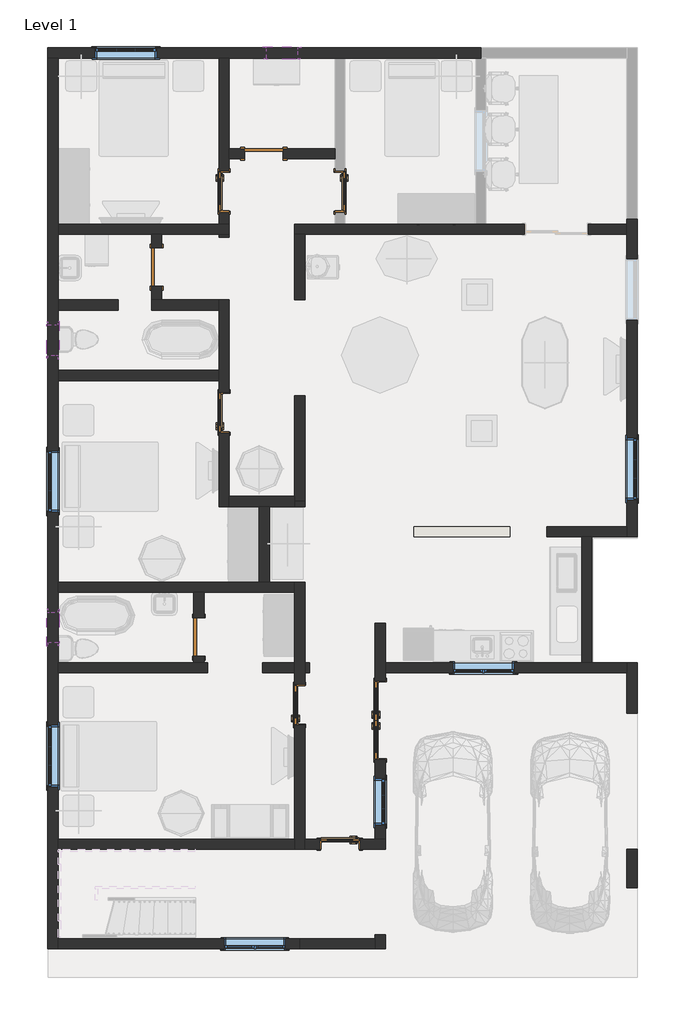
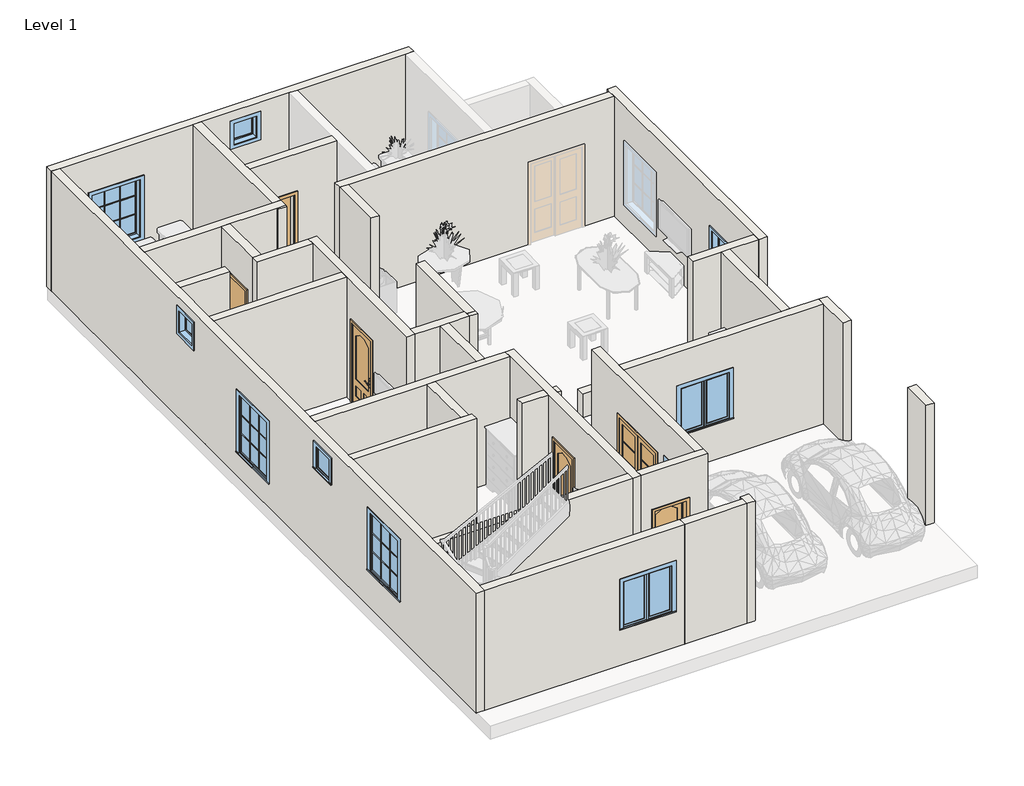
# One storey, part 1 of 3: 36 walls, 10 windows, 9 doors.
"""IFC4 building model written with IfcOpenShell, lengths in millimetres."""

from ifc_helpers import new_model, si_unit, frame, origin, origin_with_axes, place, context, project, spatial, polyline, outline, extrude, faceted_brep, transform, mapped, element, save
from components import door_ad59dcae, door_41326d50, door_b03bd389, door_53b1b562, door_fadea3f2, window_29c06734, window_cfa1ffdd, window_0862ab64, window_e41d21a6

model = new_model("IFC4")

# Units and contexts
model_context = context("Model", 3, world=origin())
ifc_project = project(units=[si_unit("LENGTHUNIT", "METRE", prefix="MILLI")], contexts=[model_context])

# Site, building, storey
site = spatial("IfcSite", under=ifc_project)
building = spatial("IfcBuilding", under=site)
storey = spatial("IfcBuildingStorey", under=building, Name="Level 1", Elevation=0.0)

# Doors
placement = place(None, origin())
door_shape = door_ad59dcae(model_context)
element("IfcDoor", 1, ObjectType="30\" x 80\"", at=placement, inside=storey, context=model_context, shape_type="MappedRepresentation", body=[
    mapped(door_shape, transform((-7772.131213, -1797.5616944, 0.0), x_axis=(1.0, 0.0, 0.0), y_axis=(0.0, 1.0, 0.0), z_axis=(0.0, 0.0, 1.0))),
])
element("IfcDoor", 2, ObjectType="30\" x 80\"", at=placement, inside=storey, context=model_context, shape_type="MappedRepresentation", body=[
    mapped(door_shape, transform((-10075.306213, 11149.2633056, 0.0), x_axis=(0.0, 1.0, 0.0), y_axis=(-1.0, 0.0, 0.0), z_axis=(0.0, 0.0, 1.0))),
])
door_2_shape = door_41326d50(model_context)
element("IfcDoor", 3, ObjectType="30\" x 80\"", at=placement, inside=storey, context=model_context, shape_type="MappedRepresentation", body=[
    mapped(door_2_shape, transform((-8575.306213, 962.6633056, 0.0), x_axis=(0.0, -1.0, 0.0), y_axis=(1.0, 0.0, 0.0), z_axis=(0.0, 0.0, 1.0))),
])
element("IfcDoor", 4, ObjectType="30\" x 80\"", at=placement, inside=storey, context=model_context, shape_type="MappedRepresentation", body=[
    mapped(door_2_shape, transform((-10075.306213, 6762.6633056, 0.0), x_axis=(0.0, -1.0, 0.0), y_axis=(1.0, 0.0, 0.0), z_axis=(0.0, 0.0, 1.0))),
])
element("IfcDoor", 5, ObjectType="30\" x 80\"", at=placement, inside=storey, context=model_context, shape_type="MappedRepresentation", body=[
    mapped(door_2_shape, transform((-7768.956213, 11149.2633056, 0.0), x_axis=(0.0, 1.0, 0.0), y_axis=(-1.0, 0.0, 0.0), z_axis=(0.0, 0.0, 1.0))),
])
door_3_shape = door_b03bd389(model_context)
element("IfcDoor", 6, ObjectType="Door-Exterior-Double-Full Glass-Wood_Clad : 60\" x 80\"", at=placement, inside=storey, context=model_context, shape_type="MappedRepresentation", body=[
    mapped(door_3_shape, transform((-6975.306213, 657.8633056, 0.0), x_axis=(0.0, 1.0, 0.0), y_axis=(-1.0, 0.0, 0.0), z_axis=(0.0, 0.0, 1.0))),
])
door_4_shape = door_53b1b562(model_context)
element("IfcDoor", 7, ObjectType="Single-Flush : 30\" x 80\"", at=placement, inside=storey, context=model_context, shape_type="MappedRepresentation", body=[
    mapped(door_4_shape, transform((-10572.131213, 2308.8633056, 0.0), x_axis=(0.0, -1.0, 0.0), y_axis=(1.0, 0.0, 0.0), z_axis=(0.0, 0.0, 1.0))),
])
element("IfcDoor", 8, ObjectType="Single-Flush : 30\" x 80\"", at=placement, inside=storey, context=model_context, shape_type="MappedRepresentation", body=[
    mapped(door_4_shape, transform((-9284.731213, 11899.2633056, 0.0), x_axis=(-1.0, 0.0, 0.0), y_axis=(0.0, -1.0, 0.0), z_axis=(0.0, 0.0, 1.0))),
])
door_5_shape = door_fadea3f2(model_context)
element("IfcDoor", 9, ObjectType="Single-Flush : 30\" x 80\"", at=placement, inside=storey, context=model_context, shape_type="MappedRepresentation", body=[
    mapped(door_5_shape, transform((-11410.331213, 9649.2633056, 0.0), x_axis=(0.0, 1.0, 0.0), y_axis=(-1.0, 0.0, 0.0), z_axis=(0.0, 0.0, 1.0))),
])

# Walls
element("IfcWall", 10, ObjectType="Generic - 8\"", at=placement, inside=storey, context=model_context, shape_type="Brep", body=[
    faceted_brep([(-13573.731213, 13797.6633056, 0.0), (-13370.531213, 13797.6633056, 0.0), (-10173.731213, 13797.6633056, 0.0), (-9970.531213, 13797.6633056, 0.0), (-7873.731213, 13797.6633056, 0.0), (-7670.531213, 13797.6633056, 0.0), (-5073.731213, 13797.6633056, 0.0), (-4972.131213, 13797.6633056, 0.0), (-4972.131213, 13797.6633056, 1219.2), (-4870.531213, 13797.6633056, 1219.2), (-4870.531213, 13797.6633056, 3048.0), (-5073.731213, 13797.6633056, 3048.0), (-7670.531213, 13797.6633056, 3048.0), (-7873.731213, 13797.6633056, 3048.0), (-9970.531213, 13797.6633056, 3048.0), (-10173.731213, 13797.6633056, 3048.0), (-13370.531213, 13797.6633056, 3048.0), (-13573.731213, 13797.6633056, 3048.0), (-11414.731213, 13797.6633056, 2133.6), (-11414.731213, 13797.6633056, 609.6), (-12633.931213, 13797.6633056, 609.6), (-12633.931213, 13797.6633056, 2133.6), (-8617.331213, 13797.6633056, 2768.6), (-8617.331213, 13797.6633056, 2159.0), (-9226.931213, 13797.6633056, 2159.0), (-9226.931213, 13797.6633056, 2768.6), (-13573.731213, 14000.8633056, 0.0), (-13573.731213, 14000.8633056, 3048.0), (-4870.531213, 14000.8633056, 3048.0), (-4870.531213, 14000.8633056, 1219.2), (-4972.131213, 14000.8633056, 1219.2), (-4972.131213, 14000.8633056, 0.0), (-11414.731213, 14000.8633056, 2133.6), (-12633.931213, 14000.8633056, 2133.6), (-12633.931213, 14000.8633056, 609.6), (-11414.731213, 14000.8633056, 609.6), (-8617.331213, 14000.8633056, 2768.6), (-9226.931213, 14000.8633056, 2768.6), (-9226.931213, 14000.8633056, 2159.0), (-8617.331213, 14000.8633056, 2159.0)], [[[0, 1, 2, 3, 4, 5, 6, 7, 8, 9, 10, 11, 12, 13, 14, 15, 16, 17], [18, 19, 20, 21], [22, 23, 24, 25]], [[26, 27, 28, 29, 30, 31], [32, 33, 34, 35], [36, 37, 38, 39]], [[7, 6, 5, 4, 3, 2, 1, 0, 26, 31]], [[0, 17, 27, 26]], [[8, 7, 31, 30]], [[29, 9, 8, 30]], [[10, 9, 29, 28]], [[19, 18, 32, 35]], [[20, 19, 35, 34]], [[21, 20, 34, 33]], [[18, 21, 33, 32]], [[23, 22, 36, 39]], [[24, 23, 39, 38]], [[25, 24, 38, 37]], [[22, 25, 37, 36]], [[17, 16, 15, 14, 13, 12, 11, 10, 28, 27]]]),
])
element("IfcWall", 11, ObjectType="Generic - 8\"", at=placement, inside=storey, context=model_context, shape_type="Brep", body=[
    faceted_brep([(-13370.531213, 10297.6633056, 0.0), (-11511.931213, 10297.6633056, 0.0), (-11308.731213, 10297.6633056, 0.0), (-10173.731213, 10297.6633056, 0.0), (-9970.531213, 10297.6633056, 0.0), (-9970.531213, 10297.6633056, 3048.0), (-10173.731213, 10297.6633056, 3048.0), (-11308.731213, 10297.6633056, 3048.0), (-11511.931213, 10297.6633056, 3048.0), (-13370.531213, 10297.6633056, 3048.0), (-13370.531213, 10500.8633056, 0.0), (-13370.531213, 10500.8633056, 3048.0), (-10173.731213, 10500.8633056, 3048.0), (-9970.531213, 10500.8633056, 3048.0), (-9970.531213, 10500.8633056, 0.0), (-10173.731213, 10500.8633056, 0.0)], [[[0, 1, 2, 3, 4, 5, 6, 7, 8, 9]], [[10, 11, 12, 13, 14, 15]], [[4, 3, 2, 1, 0, 10, 15, 14]], [[0, 9, 11, 10]], [[5, 4, 14, 13]], [[9, 8, 7, 6, 5, 13, 12, 11]]]),
])
element("IfcWall", 12, ObjectType="Generic - 8\"", at=placement, inside=storey, context=model_context, shape_type="SweptSolid", body=[
    extrude(outline(polyline([(-10173.731213, 7397.6633056), (-13370.531213, 7397.6633056), (-13370.531213, 7600.8633056), (-10173.731213, 7600.8633056), (-10173.731213, 7397.6633056)])), origin_with_axes(), (0.0, 0.0, 1.0), 3048.0),
])
element("IfcWall", 13, ObjectType="Generic - 8\"", at=placement, inside=storey, context=model_context, shape_type="Brep", body=[
    faceted_brep([(-13370.531213, 3197.6633056, 0.0), (-10673.731213, 3197.6633056, 0.0), (-10470.531213, 3197.6633056, 0.0), (-8673.731213, 3197.6633056, 0.0), (-8673.731213, 3197.6633056, 3048.0), (-10470.531213, 3197.6633056, 3048.0), (-10673.731213, 3197.6633056, 3048.0), (-13370.531213, 3197.6633056, 3048.0), (-13370.531213, 3400.8633056, 0.0), (-13370.531213, 3400.8633056, 3048.0), (-9373.731213, 3400.8633056, 3048.0), (-9170.531213, 3400.8633056, 3048.0), (-8673.731213, 3400.8633056, 3048.0), (-8673.731213, 3400.8633056, 0.0), (-9170.531213, 3400.8633056, 0.0), (-9373.731213, 3400.8633056, 0.0)], [[[0, 1, 2, 3, 4, 5, 6, 7]], [[8, 9, 10, 11, 12, 13, 14, 15]], [[3, 2, 1, 0, 8, 15, 14, 13]], [[0, 7, 9, 8]], [[4, 3, 13, 12]], [[7, 6, 5, 4, 12, 11, 10, 9]]]),
])
element("IfcWall", 14, ObjectType="Generic - 8\"", at=placement, inside=storey, context=model_context, shape_type="SweptSolid", body=[
    extrude(outline(polyline([(0.0, -13370.531213), (0.0, -8572.131213), (3048.0, -8572.131213), (3048.0, -13370.531213), (0.0, -13370.531213)]), holes=[polyline([(2133.6, -10070.731213), (2133.6, -8851.531213), (914.4, -8851.531213), (914.4, -10070.731213), (2133.6, -10070.731213)])]), frame((0.0, -3878.5366944, 0.0), z_axis=(0.0, 1.0, 0.0), x_axis=(0.0, 0.0, 1.0)), (0.0, 0.0, 1.0), 203.2),
])
element("IfcWall", 15, ObjectType="Generic - 8\"", at=placement, inside=storey, context=model_context, shape_type="SweptSolid", body=[
    extrude(outline(polyline([(-8673.731213, 8999.2633056), (-8673.731213, 10297.6633056), (-8470.531213, 10297.6633056), (-8470.531213, 8999.2633056), (-8673.731213, 8999.2633056)])), origin_with_axes(), (0.0, 0.0, 1.0), 3048.0),
])
element("IfcWall", 16, ObjectType="Generic - 8\"", at=placement, inside=storey, context=model_context, shape_type="Brep", body=[
    faceted_brep([(-9970.531213, 10500.8633056, 3048.0), (-9970.531213, 10500.8633056, 0.0), (-9970.531213, 10742.8633056, 0.0), (-9970.531213, 10742.8633056, 2057.4), (-9970.531213, 11555.6633056, 2057.4), (-9970.531213, 11555.6633056, 0.0), (-9970.531213, 11797.6633056, 0.0), (-9970.531213, 12000.8633056, 0.0), (-9970.531213, 13797.6633056, 0.0), (-9970.531213, 13797.6633056, 3048.0), (-9970.531213, 12000.8633056, 3048.0), (-9970.531213, 11797.6633056, 3048.0), (-10173.731213, 10500.8633056, 0.0), (-10173.731213, 10500.8633056, 3048.0), (-10173.731213, 13797.6633056, 3048.0), (-10173.731213, 13797.6633056, 0.0), (-10173.731213, 11555.6633056, 0.0), (-10173.731213, 11555.6633056, 2057.4), (-10173.731213, 10742.8633056, 2057.4), (-10173.731213, 10742.8633056, 0.0)], [[[0, 1, 2, 3, 4, 5, 6, 7, 8, 9, 10, 11]], [[12, 13, 14, 15, 16, 17, 18, 19]], [[1, 12, 19, 2]], [[15, 8, 7, 6, 5, 16]], [[1, 0, 13, 12]], [[9, 8, 15, 14]], [[4, 17, 16, 5]], [[17, 4, 3, 18]], [[18, 3, 2, 19]], [[0, 11, 10, 9, 14, 13]]]),
])
element("IfcWall", 17, ObjectType="Generic - 8\"", at=placement, inside=storey, context=model_context, shape_type="SweptSolid", body=[
    extrude(outline(polyline([(0.0, -9970.531213), (0.0, -9665.731213), (2032.0, -9665.731213), (2032.0, -8903.731213), (0.0, -8903.731213), (0.0, -7873.731213), (3048.0, -7873.731213), (3048.0, -9970.531213), (0.0, -9970.531213)])), frame((0.0, 11797.6633056, 0.0), z_axis=(0.0, 1.0, 0.0), x_axis=(0.0, 0.0, 1.0)), (0.0, 0.0, 1.0), 203.2),
])
element("IfcWall", 18, ObjectType="Generic - 8\"", at=placement, inside=storey, context=model_context, shape_type="Brep", body=[
    faceted_brep([(-8673.731213, 10297.6633056, 3048.0), (-8673.731213, 10297.6633056, 0.0), (-8470.531213, 10297.6633056, 0.0), (-4107.131213, 10297.6633056, 0.0), (-4107.131213, 10297.6633056, 2057.4), (-2837.131213, 10297.6633056, 2057.4), (-2837.131213, 10297.6633056, 0.0), (-2073.731213, 10297.6633056, 0.0), (-2073.731213, 10297.6633056, 3048.0), (-8470.531213, 10297.6633056, 3048.0), (-8673.731213, 10500.8633056, 0.0), (-8673.731213, 10500.8633056, 3048.0), (-7873.731213, 10500.8633056, 3048.0), (-7670.531213, 10500.8633056, 3048.0), (-5073.731213, 10500.8633056, 3048.0), (-4870.531213, 10500.8633056, 3048.0), (-2073.731213, 10500.8633056, 3048.0), (-2073.731213, 10500.8633056, 0.0), (-2837.131213, 10500.8633056, 0.0), (-2837.131213, 10500.8633056, 2057.4), (-4107.131213, 10500.8633056, 2057.4), (-4107.131213, 10500.8633056, 0.0), (-4870.531213, 10500.8633056, 0.0), (-5073.731213, 10500.8633056, 0.0), (-7670.531213, 10500.8633056, 0.0), (-7873.731213, 10500.8633056, 0.0)], [[[0, 1, 2, 3, 4, 5, 6, 7, 8, 9]], [[10, 11, 12, 13, 14, 15, 16, 17, 18, 19, 20, 21, 22, 23, 24, 25]], [[1, 10, 25, 24, 23, 22, 21, 3, 2]], [[17, 7, 6, 18]], [[1, 0, 11, 10]], [[8, 7, 17, 16]], [[20, 4, 3, 21]], [[4, 20, 19, 5]], [[5, 19, 18, 6]], [[0, 9, 8, 16, 15, 14, 13, 12, 11]]]),
])
element("IfcWall", 19, ObjectType="Generic - 8\"", at=placement, inside=storey, context=model_context, shape_type="SweptSolid", body=[
    extrude(outline(polyline([(-10173.731213, 10246.8633056), (-10173.731213, 10297.6633056), (-9970.531213, 10297.6633056), (-9970.531213, 10246.8633056), (-10173.731213, 10246.8633056)])), origin_with_axes(), (0.0, 0.0, 1.0), 3048.0),
])
element("IfcWall", 20, ObjectType="Generic - 8\"", at=placement, inside=storey, context=model_context, shape_type="Brep", body=[
    faceted_brep([(-10173.731213, 9000.8633056, 0.0), (-11308.731213, 9000.8633056, 0.0), (-11511.931213, 9000.8633056, 0.0), (-11511.931213, 9000.8633056, 3048.0), (-11308.731213, 9000.8633056, 3048.0), (-10173.731213, 9000.8633056, 3048.0), (-10173.731213, 8797.6633056, 0.0), (-10173.731213, 8797.6633056, 3048.0), (-11511.931213, 8797.6633056, 3048.0), (-11511.931213, 8797.6633056, 0.0)], [[[0, 1, 2, 3, 4, 5]], [[6, 7, 8, 9]], [[2, 1, 0, 6, 9]], [[3, 2, 9, 8]], [[0, 5, 7, 6]], [[5, 4, 3, 8, 7]]]),
])
element("IfcWall", 21, ObjectType="Generic - 8\"", at=placement, inside=storey, context=model_context, shape_type="SweptSolid", body=[
    extrude(outline(polyline([(-9170.531213, 4897.6633056), (-9170.531213, 3400.8633056), (-9373.731213, 3400.8633056), (-9373.731213, 4897.6633056), (-9170.531213, 4897.6633056)])), origin_with_axes(), (0.0, 0.0, 1.0), 3048.0),
])
element("IfcWall", 22, ObjectType="Generic - 8\"", at=placement, inside=storey, context=model_context, shape_type="Brep", body=[
    faceted_brep([(-9970.531213, 4897.6633056, 0.0), (-9373.731213, 4897.6633056, 0.0), (-9170.531213, 4897.6633056, 0.0), (-8673.731213, 4897.6633056, 0.0), (-8673.731213, 4897.6633056, 3048.0), (-9170.531213, 4897.6633056, 3048.0), (-9373.731213, 4897.6633056, 3048.0), (-9970.531213, 4897.6633056, 3048.0), (-9970.531213, 5100.8633056, 0.0), (-9970.531213, 5100.8633056, 3048.0), (-8673.731213, 5100.8633056, 3048.0), (-8673.731213, 5100.8633056, 0.0), (-8673.731213, 4999.2633056, 0.0), (-8673.731213, 4899.2633056, 0.0), (-8673.731213, 4999.2633056, 3048.0), (-8673.731213, 4899.2633056, 3048.0)], [[[0, 1, 2, 3, 4, 5, 6, 7]], [[8, 9, 10, 11]], [[3, 2, 1, 0, 8, 11, 12, 13]], [[4, 3, 13, 12, 11, 10, 14, 15]], [[0, 7, 9, 8]], [[7, 6, 5, 4, 15, 14, 10, 9]]]),
])
element("IfcWall", 23, ObjectType="Generic - 8\"", at=placement, inside=storey, context=model_context, shape_type="SweptSolid", body=[
    extrude(outline(polyline([(-8673.731213, 4899.2633056), (-8673.731213, 4999.2633056), (-8470.531213, 4999.2633056), (-8470.531213, 4899.2633056), (-8673.731213, 4899.2633056)])), origin_with_axes(), (0.0, 0.0, 1.0), 3048.0),
])
element("IfcWall", 24, ObjectType="Generic - 8\"", at=placement, inside=storey, context=model_context, shape_type="Brep", body=[
    faceted_brep([(-8673.731213, 3400.8633056, 3048.0), (-8673.731213, 3400.8633056, 0.0), (-8673.731213, 3197.6633056, 0.0), (-8673.731213, 1800.8633056, 0.0), (-8673.731213, 1597.6633056, 0.0), (-8673.731213, 1369.0633056, 0.0), (-8673.731213, 1369.0633056, 2057.4), (-8673.731213, 556.2633056, 2057.4), (-8673.731213, 556.2633056, 0.0), (-8673.731213, -1699.1366944, 0.0), (-8673.731213, -1902.3366944, 0.0), (-8673.731213, -1902.3366944, 3048.0), (-8673.731213, -1699.1366944, 3048.0), (-8673.731213, 1597.6633056, 3048.0), (-8673.731213, 1800.8633056, 3048.0), (-8673.731213, 3197.6633056, 3048.0), (-8470.531213, 3400.8633056, 0.0), (-8470.531213, 3400.8633056, 3048.0), (-8470.531213, 1800.8633056, 3048.0), (-8470.531213, 1597.6633056, 3048.0), (-8470.531213, -1699.1366944, 3048.0), (-8470.531213, -1902.3366944, 3048.0), (-8470.531213, -1902.3366944, 0.0), (-8470.531213, -1699.1366944, 0.0), (-8470.531213, 556.2633056, 0.0), (-8470.531213, 556.2633056, 2057.4), (-8470.531213, 1369.0633056, 2057.4), (-8470.531213, 1369.0633056, 0.0), (-8470.531213, 1597.6633056, 0.0), (-8470.531213, 1800.8633056, 0.0)], [[[0, 1, 2, 3, 4, 5, 6, 7, 8, 9, 10, 11, 12, 13, 14, 15]], [[16, 17, 18, 19, 20, 21, 22, 23, 24, 25, 26, 27, 28, 29]], [[1, 16, 29, 28, 27, 5, 4, 3, 2]], [[22, 10, 9, 8, 24, 23]], [[1, 0, 17, 16]], [[11, 10, 22, 21]], [[7, 25, 24, 8]], [[25, 7, 6, 26]], [[26, 6, 5, 27]], [[0, 15, 14, 13, 12, 11, 21, 20, 19, 18, 17]]]),
])
element("IfcWall", 25, ObjectType="Generic - 8\"", at=placement, inside=storey, context=model_context, shape_type="SweptSolid", body=[
    extrude(outline(polyline([(-9308.731213, 1800.8633056), (-8673.731213, 1800.8633056), (-8673.731213, 1597.6633056), (-9308.731213, 1597.6633056), (-9308.731213, 1800.8633056)])), origin_with_axes(), (0.0, 0.0, 1.0), 3048.0),
])
element("IfcWall", 26, ObjectType="Generic - 8\"", at=placement, inside=storey, context=model_context, shape_type="SweptSolid", body=[
    extrude(outline(polyline([(1927.8633056, 2032.0), (1927.8633056, 0.0), (1800.8633056, 0.0), (1800.8633056, 3048.0), (3197.6633056, 3048.0), (3197.6633056, 0.0), (2689.8633056, 0.0), (2689.8633056, 2032.0), (1927.8633056, 2032.0)])), frame((-10673.731213, 0.0, 0.0), z_axis=(1.0, 0.0, 0.0), x_axis=(0.0, 1.0, 0.0)), (0.0, 0.0, 1.0), 203.2),
])
element("IfcWall", 27, ObjectType="Generic - 8\"", at=placement, inside=storey, context=model_context, shape_type="SweptSolid", body=[
    extrude(outline(polyline([(-13370.531213, -1699.1366944), (-8673.731213, -1699.1366944), (-8673.731213, -1902.3366944), (-13370.531213, -1902.3366944), (-13370.531213, -1699.1366944)])), origin_with_axes(), (0.0, 0.0, 1.0), 3048.0),
])
element("IfcWall", 28, ObjectType="Generic - 8\"", at=placement, inside=storey, context=model_context, shape_type="SweptSolid", body=[
    extrude(outline(polyline([(-8372.131213, 1597.6633056), (-8470.531213, 1597.6633056), (-8470.531213, 1800.8633056), (-8372.131213, 1800.8633056), (-8372.131213, 1597.6633056)])), origin_with_axes(), (0.0, 0.0, 1.0), 3048.0),
])
element("IfcWall", 29, ObjectType="Generic - 8\"", at=placement, inside=storey, context=model_context, shape_type="Brep", body=[
    faceted_brep([(-7073.731213, 2580.2633056, 3048.0), (-7073.731213, 2580.2633056, 0.0), (-7073.731213, 1445.2633056, 0.0), (-7073.731213, 1445.2633056, 2057.4), (-7073.731213, -129.5366944, 2057.4), (-7073.731213, -129.5366944, 0.0), (-7073.731213, -1699.1366944, 0.0), (-7073.731213, -1699.1366944, 3048.0), (-7073.731213, -1419.7366944, 2133.6), (-7073.731213, -1419.7366944, 914.4), (-7073.731213, -505.3366944, 914.4), (-7073.731213, -505.3366944, 2133.6), (-6870.531213, 2580.2633056, 0.0), (-6870.531213, 2580.2633056, 3048.0), (-6870.531213, 1800.8633056, 3048.0), (-6870.531213, 1597.6633056, 3048.0), (-6870.531213, -1699.1366944, 3048.0), (-6870.531213, -1699.1366944, 0.0), (-6870.531213, -129.5366944, 0.0), (-6870.531213, -129.5366944, 2057.4), (-6870.531213, 1445.2633056, 2057.4), (-6870.531213, 1445.2633056, 0.0), (-6870.531213, 1597.6633056, 0.0), (-6870.531213, 1800.8633056, 0.0), (-6870.531213, -1419.7366944, 2133.6), (-6870.531213, -505.3366944, 2133.6), (-6870.531213, -505.3366944, 914.4), (-6870.531213, -1419.7366944, 914.4)], [[[0, 1, 2, 3, 4, 5, 6, 7], [8, 9, 10, 11]], [[12, 13, 14, 15, 16, 17, 18, 19, 20, 21, 22, 23], [24, 25, 26, 27]], [[1, 12, 23, 22, 21, 2]], [[17, 6, 5, 18]], [[1, 0, 13, 12]], [[7, 6, 17, 16]], [[20, 3, 2, 21]], [[3, 20, 19, 4]], [[4, 19, 18, 5]], [[9, 8, 24, 27]], [[10, 9, 27, 26]], [[11, 10, 26, 25]], [[8, 11, 25, 24]], [[0, 7, 16, 15, 14, 13]]]),
])
element("IfcWall", 30, ObjectType="Generic - 8\"", at=placement, inside=storey, context=model_context, shape_type="SweptSolid", body=[
    extrude(outline(polyline([(-8572.131213, -3675.3366944), (-7073.731213, -3675.3366944), (-7073.731213, -3878.5366944), (-8572.131213, -3878.5366944), (-8572.131213, -3675.3366944)])), origin_with_axes(), (0.0, 0.0, 1.0), 3048.0),
])
element("IfcWall", 31, ObjectType="Generic - 8\"", at=placement, inside=storey, context=model_context, shape_type="Brep", body=[
    faceted_brep([(-13370.531213, -3878.5366944, 0.0), (-13370.531213, -3675.3366944, 0.0), (-13370.531213, -1902.3366944, 0.0), (-13370.531213, -1699.1366944, 0.0), (-13370.531213, 1597.6633056, 0.0), (-13370.531213, 1800.8633056, 0.0), (-13370.531213, 3197.6633056, 0.0), (-13370.531213, 3400.8633056, 0.0), (-13370.531213, 7397.6633056, 0.0), (-13370.531213, 7600.8633056, 0.0), (-13370.531213, 8797.6633056, 0.0), (-13370.531213, 9000.8633056, 0.0), (-13370.531213, 10297.6633056, 0.0), (-13370.531213, 10500.8633056, 0.0), (-13370.531213, 13797.6633056, 0.0), (-13370.531213, 13797.6633056, 3048.0), (-13370.531213, 10500.8633056, 3048.0), (-13370.531213, 10297.6633056, 3048.0), (-13370.531213, 9000.8633056, 3048.0), (-13370.531213, 8797.6633056, 3048.0), (-13370.531213, 7600.8633056, 3048.0), (-13370.531213, 7397.6633056, 3048.0), (-13370.531213, 3400.8633056, 3048.0), (-13370.531213, 3197.6633056, 3048.0), (-13370.531213, 1800.8633056, 3048.0), (-13370.531213, 1597.6633056, 3048.0), (-13370.531213, -1699.1366944, 3048.0), (-13370.531213, -1902.3366944, 3048.0), (-13370.531213, -3675.3366944, 3048.0), (-13370.531213, -3878.5366944, 3048.0), (-13370.531213, 558.8633056, 2438.4), (-13370.531213, 558.8633056, 914.4), (-13370.531213, -660.3366944, 914.4), (-13370.531213, -660.3366944, 2438.4), (-13370.531213, 6008.8633056, 2133.6), (-13370.531213, 6008.8633056, 609.6), (-13370.531213, 4789.6633056, 609.6), (-13370.531213, 4789.6633056, 2133.6), (-13370.531213, 2804.0633056, 2768.6), (-13370.531213, 2804.0633056, 2159.0), (-13370.531213, 2194.4633056, 2159.0), (-13370.531213, 2194.4633056, 2768.6), (-13370.531213, 7894.4633056, 2768.6), (-13370.531213, 8504.0633056, 2768.6), (-13370.531213, 8504.0633056, 2159.0), (-13370.531213, 7894.4633056, 2159.0), (-13573.731213, -3878.5366944, 0.0), (-13573.731213, -3878.5366944, 3048.0), (-13573.731213, 13797.6633056, 3048.0), (-13573.731213, 13797.6633056, 0.0), (-13573.731213, 558.8633056, 2438.4), (-13573.731213, -660.3366944, 2438.4), (-13573.731213, -660.3366944, 914.4), (-13573.731213, 558.8633056, 914.4), (-13573.731213, 6008.8633056, 2133.6), (-13573.731213, 4789.6633056, 2133.6), (-13573.731213, 4789.6633056, 609.6), (-13573.731213, 6008.8633056, 609.6), (-13573.731213, 2804.0633056, 2768.6), (-13573.731213, 2194.4633056, 2768.6), (-13573.731213, 2194.4633056, 2159.0), (-13573.731213, 2804.0633056, 2159.0), (-13573.731213, 7894.4633056, 2768.6), (-13573.731213, 7894.4633056, 2159.0), (-13573.731213, 8504.0633056, 2159.0), (-13573.731213, 8504.0633056, 2768.6)], [[[0, 1, 2, 3, 4, 5, 6, 7, 8, 9, 10, 11, 12, 13, 14, 15, 16, 17, 18, 19, 20, 21, 22, 23, 24, 25, 26, 27, 28, 29], [30, 31, 32, 33], [34, 35, 36, 37], [38, 39, 40, 41], [42, 43, 44, 45]], [[46, 47, 48, 49], [50, 51, 52, 53], [54, 55, 56, 57], [58, 59, 60, 61], [62, 63, 64, 65]], [[14, 13, 12, 11, 10, 9, 8, 7, 6, 5, 4, 3, 2, 1, 0, 46, 49]], [[15, 14, 49, 48]], [[0, 29, 47, 46]], [[31, 30, 50, 53]], [[32, 31, 53, 52]], [[33, 32, 52, 51]], [[30, 33, 51, 50]], [[35, 34, 54, 57]], [[36, 35, 57, 56]], [[37, 36, 56, 55]], [[34, 37, 55, 54]], [[39, 38, 58, 61]], [[40, 39, 61, 60]], [[41, 40, 60, 59]], [[38, 41, 59, 58]], [[63, 62, 42, 45]], [[64, 63, 45, 44]], [[65, 64, 44, 43]], [[62, 65, 43, 42]], [[29, 28, 27, 26, 25, 24, 23, 22, 21, 20, 19, 18, 17, 16, 15, 48, 47]]]),
])
element("IfcWall", 32, ObjectType="Generic - 8\"", at=placement, inside=storey, context=model_context, shape_type="Brep", body=[
    faceted_brep([(-7073.731213, -3600.7366944, 0.0), (-7073.731213, -3675.3366944, 0.0), (-7073.731213, -3878.5366944, 0.0), (-7073.731213, -3878.5366944, 3048.0), (-7073.731213, -3675.3366944, 3048.0), (-7073.731213, -3600.7366944, 3048.0), (-6870.531213, -3600.7366944, 0.0), (-6870.531213, -3600.7366944, 3048.0), (-6870.531213, -3878.5366944, 3048.0), (-6870.531213, -3878.5366944, 0.0)], [[[0, 1, 2, 3, 4, 5]], [[6, 7, 8, 9]], [[2, 1, 0, 6, 9]], [[0, 5, 7, 6]], [[3, 2, 9, 8]], [[5, 4, 3, 8, 7]]]),
])
element("IfcWall", 33, ObjectType="Generic - 8\"", at=placement, inside=storey, context=model_context, shape_type="Brep", body=[
    faceted_brep([(-6870.531213, -1902.3366944, 0.0), (-6870.531213, -1902.3366944, 3048.0), (-8470.531213, -1902.3366944, 3048.0), (-8470.531213, -1902.3366944, 0.0), (-8178.531213, -1902.3366944, 0.0), (-8178.531213, -1902.3366944, 2057.4), (-7365.731213, -1902.3366944, 2057.4), (-7365.731213, -1902.3366944, 0.0), (-6870.531213, -1699.1366944, 3048.0), (-6870.531213, -1699.1366944, 0.0), (-7073.731213, -1699.1366944, 0.0), (-7365.731213, -1699.1366944, 0.0), (-7365.731213, -1699.1366944, 2057.4), (-8178.531213, -1699.1366944, 2057.4), (-8178.531213, -1699.1366944, 0.0), (-8470.531213, -1699.1366944, 0.0), (-8470.531213, -1699.1366944, 3048.0), (-7073.731213, -1699.1366944, 3048.0)], [[[0, 1, 2, 3, 4, 5, 6, 7]], [[8, 9, 10, 11, 12, 13, 14, 15, 16, 17]], [[9, 0, 7, 11, 10]], [[3, 15, 14, 4]], [[1, 0, 9, 8]], [[3, 2, 16, 15]], [[6, 12, 11, 7]], [[12, 6, 5, 13]], [[13, 5, 4, 14]], [[2, 1, 8, 17, 16]]]),
])
element("IfcWall", 34, ObjectType="Generic - 8\"", at=placement, inside=storey, context=model_context, shape_type="Brep", body=[
    faceted_brep([(-6870.531213, 1597.6633056, 0.0), (-2073.731213, 1597.6633056, 0.0), (-2073.731213, 1597.6633056, 3048.0), (-6870.531213, 1597.6633056, 3048.0), (-5531.731213, 1597.6633056, 2133.6), (-4312.531213, 1597.6633056, 2133.6), (-4312.531213, 1597.6633056, 914.4), (-5531.731213, 1597.6633056, 914.4), (-6870.531213, 1800.8633056, 0.0), (-6870.531213, 1800.8633056, 3048.0), (-2973.731213, 1800.8633056, 3048.0), (-2770.531213, 1800.8633056, 3048.0), (-2073.731213, 1800.8633056, 3048.0), (-2073.731213, 1800.8633056, 0.0), (-2770.531213, 1800.8633056, 0.0), (-2973.731213, 1800.8633056, 0.0), (-5531.731213, 1800.8633056, 2133.6), (-5531.731213, 1800.8633056, 914.4), (-4312.531213, 1800.8633056, 914.4), (-4312.531213, 1800.8633056, 2133.6), (-2073.731213, 1799.2633056, 0.0), (-2073.731213, 1799.2633056, 3048.0)], [[[0, 1, 2, 3], [4, 5, 6, 7]], [[8, 9, 10, 11, 12, 13, 14, 15], [16, 17, 18, 19]], [[1, 0, 8, 15, 14, 13, 20]], [[2, 1, 20, 13, 12, 21]], [[0, 3, 9, 8]], [[17, 16, 4, 7]], [[18, 17, 7, 6]], [[19, 18, 6, 5]], [[16, 19, 5, 4]], [[3, 2, 21, 12, 11, 10, 9]]]),
])
element("IfcWall", 35, ObjectType="Generic - 8\"", at=placement, inside=storey, context=model_context, shape_type="SweptSolid", body=[
    extrude(outline(polyline([(-2770.531213, 4297.6633056), (-2770.531213, 1800.8633056), (-2973.731213, 1800.8633056), (-2973.731213, 4297.6633056), (-2770.531213, 4297.6633056)])), origin_with_axes(), (0.0, 0.0, 1.0), 3048.0),
])
element("IfcWall", 36, ObjectType="Generic - 8\"", at=placement, inside=storey, context=model_context, shape_type="Brep", body=[
    faceted_brep([(-2073.731213, 1799.2633056, 0.0), (-2073.731213, 1597.6633056, 0.0), (-2073.731213, 799.2633056, 0.0), (-2073.731213, 799.2633056, 3048.0), (-2073.731213, 1597.6633056, 3048.0), (-2073.731213, 1799.2633056, 3048.0), (-1870.531213, 1799.2633056, 0.0), (-1870.531213, 1799.2633056, 3048.0), (-1870.531213, 799.2633056, 3048.0), (-1870.531213, 799.2633056, 0.0)], [[[0, 1, 2, 3, 4, 5]], [[6, 7, 8, 9]], [[2, 1, 0, 6, 9]], [[3, 2, 9, 8]], [[0, 5, 7, 6]], [[5, 4, 3, 8, 7]]]),
])
element("IfcWall", 37, ObjectType="Generic - 8\"", at=placement, inside=storey, context=model_context, shape_type="SweptSolid", body=[
    extrude(outline(polyline([(-2073.731213, -2662.7366944), (-2073.731213, -1900.7366944), (-1870.531213, -1900.7366944), (-1870.531213, -2662.7366944), (-2073.731213, -2662.7366944)])), origin_with_axes(), (0.0, 0.0, 1.0), 3048.0),
])
element("IfcWall", 38, ObjectType="Generic - 8\"", at=placement, inside=storey, context=model_context, shape_type="Brep", body=[
    faceted_brep([(-8673.731213, 7099.2633056, 0.0), (-8673.731213, 5100.8633056, 0.0), (-8673.731213, 4999.2633056, 0.0), (-8673.731213, 4999.2633056, 3048.0), (-8673.731213, 5100.8633056, 3048.0), (-8673.731213, 7099.2633056, 3048.0), (-8470.531213, 7099.2633056, 0.0), (-8470.531213, 7099.2633056, 3048.0), (-8470.531213, 4999.2633056, 3048.0), (-8470.531213, 4999.2633056, 0.0)], [[[0, 1, 2, 3, 4, 5]], [[6, 7, 8, 9]], [[2, 1, 0, 6, 9]], [[3, 2, 9, 8]], [[0, 5, 7, 6]], [[5, 4, 3, 8, 7]]]),
])
element("IfcWall", 39, ObjectType="Generic - 8\"", at=placement, inside=storey, context=model_context, shape_type="Brep", body=[
    faceted_brep([(-2073.731213, 10597.2633056, 0.0), (-2073.731213, 10500.8633056, 0.0), (-2073.731213, 10297.6633056, 0.0), (-2073.731213, 4500.8633056, 0.0), (-2073.731213, 4297.6633056, 0.0), (-2073.731213, 4297.6633056, 3048.0), (-2073.731213, 4500.8633056, 3048.0), (-2073.731213, 10297.6633056, 3048.0), (-2073.731213, 10500.8633056, 3048.0), (-2073.731213, 10597.2633056, 3048.0), (-2073.731213, 10597.2633056, 1219.2), (-2073.731213, 8595.8633056, 2133.6), (-2073.731213, 8595.8633056, 609.6), (-2073.731213, 9815.0633056, 609.6), (-2073.731213, 9815.0633056, 2133.6), (-2073.731213, 5034.2633056, 2133.6), (-2073.731213, 5034.2633056, 609.6), (-2073.731213, 6253.4633056, 609.6), (-2073.731213, 6253.4633056, 2133.6), (-1870.531213, 10597.2633056, 0.0), (-1870.531213, 10597.2633056, 1219.2), (-1870.531213, 10597.2633056, 3048.0), (-1870.531213, 4297.6633056, 3048.0), (-1870.531213, 4297.6633056, 0.0), (-1870.531213, 8595.8633056, 2133.6), (-1870.531213, 9815.0633056, 2133.6), (-1870.531213, 9815.0633056, 609.6), (-1870.531213, 8595.8633056, 609.6), (-1870.531213, 5034.2633056, 2133.6), (-1870.531213, 6253.4633056, 2133.6), (-1870.531213, 6253.4633056, 609.6), (-1870.531213, 5034.2633056, 609.6)], [[[0, 1, 2, 3, 4, 5, 6, 7, 8, 9, 10], [11, 12, 13, 14], [15, 16, 17, 18]], [[19, 20, 21, 22, 23], [24, 25, 26, 27], [28, 29, 30, 31]], [[4, 3, 2, 1, 0, 19, 23]], [[0, 10, 9, 21, 20, 19]], [[5, 4, 23, 22]], [[12, 11, 24, 27]], [[13, 12, 27, 26]], [[14, 13, 26, 25]], [[11, 14, 25, 24]], [[16, 15, 28, 31]], [[17, 16, 31, 30]], [[18, 17, 30, 29]], [[15, 18, 29, 28]], [[9, 8, 7, 6, 5, 22, 21]]]),
])
element("IfcWall", 40, ObjectType="Generic - 8\"", at=placement, inside=storey, context=model_context, shape_type="SweptSolid", body=[
    extrude(outline(polyline([(-6301.131213, 4500.8633056), (-4396.131213, 4500.8633056), (-4396.131213, 4297.6633056), (-6301.131213, 4297.6633056), (-6301.131213, 4500.8633056)])), origin_with_axes(), (0.0, 0.0, 1.0), 609.6),
])
element("IfcWall", 41, ObjectType="Generic - 8\"", at=placement, inside=storey, context=model_context, shape_type="Brep", body=[
    faceted_brep([(-3659.531213, 4297.6633056, 0.0), (-2973.731213, 4297.6633056, 0.0), (-2770.531213, 4297.6633056, 0.0), (-2073.731213, 4297.6633056, 0.0), (-2073.731213, 4297.6633056, 3048.0), (-2770.531213, 4297.6633056, 3048.0), (-2973.731213, 4297.6633056, 3048.0), (-3659.531213, 4297.6633056, 3048.0), (-3659.531213, 4500.8633056, 0.0), (-3659.531213, 4500.8633056, 3048.0), (-2073.731213, 4500.8633056, 3048.0), (-2073.731213, 4500.8633056, 0.0)], [[[0, 1, 2, 3, 4, 5, 6, 7]], [[8, 9, 10, 11]], [[3, 2, 1, 0, 8, 11]], [[0, 7, 9, 8]], [[4, 3, 11, 10]], [[7, 6, 5, 4, 10, 9]]]),
])
element("IfcWall", 42, ObjectType="Generic - 8\"", at=placement, inside=storey, context=model_context, shape_type="SweptSolid", body=[
    extrude(outline(polyline([(10297.6633056, 0.0), (10030.2633056, 0.0), (10030.2633056, 2032.0), (9268.2633056, 2032.0), (9268.2633056, 0.0), (9000.8633056, 0.0), (9000.8633056, 3048.0), (10297.6633056, 3048.0), (10297.6633056, 0.0)])), frame((-11511.931213, 0.0, 0.0), z_axis=(1.0, 0.0, 0.0), x_axis=(0.0, 1.0, 0.0)), (0.0, 0.0, 1.0), 203.2),
])
element("IfcWall", 43, ObjectType="Generic - 8\"", at=placement, inside=storey, context=model_context, shape_type="Brep", body=[
    faceted_brep([(-10173.731213, 9000.8633056, 3048.0), (-10173.731213, 9000.8633056, 0.0), (-10173.731213, 8797.6633056, 0.0), (-10173.731213, 7600.8633056, 0.0), (-10173.731213, 7397.6633056, 0.0), (-10173.731213, 7169.0633056, 0.0), (-10173.731213, 7169.0633056, 2057.4), (-10173.731213, 6356.2633056, 2057.4), (-10173.731213, 6356.2633056, 0.0), (-10173.731213, 4897.6633056, 0.0), (-10173.731213, 4897.6633056, 3048.0), (-10173.731213, 7397.6633056, 3048.0), (-10173.731213, 7600.8633056, 3048.0), (-10173.731213, 8797.6633056, 3048.0), (-9970.531213, 9000.8633056, 0.0), (-9970.531213, 9000.8633056, 3048.0), (-9970.531213, 5100.8633056, 3048.0), (-9970.531213, 4897.6633056, 3048.0), (-9970.531213, 4897.6633056, 0.0), (-9970.531213, 5100.8633056, 0.0), (-9970.531213, 6356.2633056, 0.0), (-9970.531213, 6356.2633056, 2057.4), (-9970.531213, 7169.0633056, 2057.4), (-9970.531213, 7169.0633056, 0.0)], [[[0, 1, 2, 3, 4, 5, 6, 7, 8, 9, 10, 11, 12, 13]], [[14, 15, 16, 17, 18, 19, 20, 21, 22, 23]], [[1, 14, 23, 5, 4, 3, 2]], [[18, 9, 8, 20, 19]], [[1, 0, 15, 14]], [[10, 9, 18, 17]], [[7, 21, 20, 8]], [[21, 7, 6, 22]], [[22, 6, 5, 23]], [[0, 13, 12, 11, 10, 17, 16, 15]]]),
])
element("IfcWall", 44, ObjectType="Generic - 8\"", at=placement, inside=storey, context=model_context, shape_type="SweptSolid", body=[
    extrude(outline(polyline([(-13370.531213, 9000.8633056), (-12180.331213, 9000.8633056), (-12180.331213, 8797.6633056), (-13370.531213, 8797.6633056), (-13370.531213, 9000.8633056)])), origin_with_axes(), (0.0, 0.0, 1.0), 3048.0),
])
element("IfcWall", 45, ObjectType="Generic - 8\"", at=placement, inside=storey, context=model_context, shape_type="Brep", body=[
    faceted_brep([(-10400.931213, 1800.8633056, 0.0), (-10470.531213, 1800.8633056, 0.0), (-10673.731213, 1800.8633056, 0.0), (-13370.531213, 1800.8633056, 0.0), (-13370.531213, 1800.8633056, 3048.0), (-10673.731213, 1800.8633056, 3048.0), (-10470.531213, 1800.8633056, 3048.0), (-10400.931213, 1800.8633056, 3048.0), (-10400.931213, 1597.6633056, 0.0), (-10400.931213, 1597.6633056, 3048.0), (-13370.531213, 1597.6633056, 3048.0), (-13370.531213, 1597.6633056, 0.0)], [[[0, 1, 2, 3, 4, 5, 6, 7]], [[8, 9, 10, 11]], [[3, 2, 1, 0, 8, 11]], [[0, 7, 9, 8]], [[4, 3, 11, 10]], [[7, 6, 5, 4, 10, 9]]]),
])

# Windows
window_shape = window_29c06734(model_context)
element("IfcWindow", 46, ObjectType="Casement 3x3 with Trim : 36\" x 48\"", at=placement, inside=storey, context=model_context, shape_type="MappedRepresentation", body=[
    mapped(window_shape, transform((-6972.131213, -962.5366944, 0.0), x_axis=(0.0, -1.0, 0.0), y_axis=(1.0, 0.0, 0.0), z_axis=(0.0, 0.0, 1.0))),
])
window_2_shape = window_cfa1ffdd(model_context)
element("IfcWindow", 47, ObjectType="Casement 3x3 with Trim : 48\" x 60\"", at=placement, inside=storey, context=model_context, shape_type="MappedRepresentation", body=[
    mapped(window_2_shape, transform((-13472.131213, -50.7366944, 304.8), x_axis=(0.0, 1.0, 0.0), y_axis=(-1.0, 0.0, 0.0), z_axis=(0.0, 0.0, 1.0))),
])
element("IfcWindow", 48, ObjectType="Casement 3x3 with Trim : 48\" x 60\"", at=placement, inside=storey, context=model_context, shape_type="MappedRepresentation", body=[
    mapped(window_2_shape, transform((-13472.131213, 5399.2633056, 0.0), x_axis=(0.0, 1.0, 0.0), y_axis=(-1.0, 0.0, 0.0), z_axis=(0.0, 0.0, 1.0))),
])
element("IfcWindow", 49, ObjectType="Casement 3x3 with Trim : 48\" x 60\"", at=placement, inside=storey, context=model_context, shape_type="MappedRepresentation", body=[
    mapped(window_2_shape, transform((-12024.331213, 13899.2633056, 0.0), x_axis=(1.0, 0.0, 0.0), y_axis=(0.0, 1.0, 0.0), z_axis=(0.0, 0.0, 1.0))),
])
element("IfcWindow", 50, ObjectType="Casement 3x3 with Trim : 48\" x 60\"", at=placement, inside=storey, context=model_context, shape_type="MappedRepresentation", body=[
    mapped(window_2_shape, transform((-1972.131213, 5643.8633056, 0.0), x_axis=(0.0, -1.0, 0.0), y_axis=(1.0, 0.0, 0.0), z_axis=(0.0, 0.0, 1.0))),
])
window_3_shape = window_0862ab64(model_context)
element("IfcWindow", 51, ObjectType="Casement Dbl with Trim : 48\" x 48\"", at=placement, inside=storey, context=model_context, shape_type="MappedRepresentation", body=[
    mapped(window_3_shape, transform((-4922.131213, 1718.3133056, 0.0), x_axis=(-1.0, 0.0, 0.0), y_axis=(0.0, -1.0, 0.0), z_axis=(0.0, 0.0, 1.0))),
])
element("IfcWindow", 52, ObjectType="Casement Dbl with Trim : 48\" x 48\"", at=placement, inside=storey, context=model_context, shape_type="MappedRepresentation", body=[
    mapped(window_3_shape, transform((-9461.131213, -3757.8866944, 0.0), x_axis=(-1.0, 0.0, 0.0), y_axis=(0.0, -1.0, 0.0), z_axis=(0.0, 0.0, 1.0))),
])
window_4_shape = window_e41d21a6(model_context)
element("IfcWindow", 53, ObjectType="Transom with Trim : 24\" x 24\"", at=placement, inside=storey, context=model_context, shape_type="MappedRepresentation", body=[
    mapped(window_4_shape, transform((-13472.131213, 2537.3633056, 0.0), x_axis=(0.0, 1.0, 0.0), y_axis=(-1.0, 0.0, 0.0), z_axis=(0.0, 0.0, 1.0))),
])
element("IfcWindow", 54, ObjectType="Transom with Trim : 24\" x 24\"", at=placement, inside=storey, context=model_context, shape_type="MappedRepresentation", body=[
    mapped(window_4_shape, transform((-13472.131213, 8161.1633056, 0.0), x_axis=(0.0, -1.0, 0.0), y_axis=(1.0, 0.0, 0.0), z_axis=(0.0, 0.0, 1.0))),
])
element("IfcWindow", 55, ObjectType="Transom with Trim : 24\" x 24\"", at=placement, inside=storey, context=model_context, shape_type="MappedRepresentation", body=[
    mapped(window_4_shape, transform((-8884.031213, 13899.2633056, 0.0), x_axis=(1.0, 0.0, 0.0), y_axis=(0.0, 1.0, 0.0), z_axis=(0.0, 0.0, 1.0))),
])

save(model, "model.ifc")

# Revit data of these elements
# Type "30\" x 80\""
#   Type Mark = "9"
#   Assembly Code = "B2030100"
#   Analytic Construction = "French door, wood frame with single glass"
#   Threshold Offset [instance default] = 0' - 0 1/2"
#   Thickness = 0' - 1 3/8"
#   Thermal Resistance (R) = 1.0696 (h·ft²·°F)/BTU
#   Swing Angle [instance default] = 90.00°
#   Stiles = 0' - 4 3/4"
#   Rough Width = 2' - 8"
#   Rough Height = 6' - 9"
#   Radius = 1' - 1.00625"
#   Lock Rail = 0' - 7 1/8"
#   Height = 6' - 8"
#   Width = 2' - 6"
#   Heat Transfer Coefficient (U) = 0.9350 BTU/(h·ft²·°F)
#   Door Offset [instance default] = 0' - 0"
#   Bottom Rail = 0' - 9 1/2"
#   Threshold [instance default] = yes
#   Function = 1
#   Exterior Trim [instance default] = yes
#   Trim Material = Cherry
#   Threshold Material = Cherry
#   Panel Material = Cherry
#   Glazing = Glass
#   Frame Material = Cherry
#   Door Handle Material = Aluminum
#   Visual Light Transmittance = 0
#   Solar Heat Gain Coefficient = 0
#   Wall Closure = (empty or 0)
#   Construction Type = (empty or 0)
# Type "Door-Exterior-Double-Full Glass-Wood_Clad : 60\" x 80\""
#   Type Mark = "8"
#   Assembly Code = "B2030100"
#   Analytic Construction = "French door, wood frame with double glass"
#   Top Rail = 0' - 4 11/16"
#   Threshold Offset [instance default] = 0' - 0 1/2"
#   Thickness = 0' - 1 3/8"
#   Thermal Resistance (R) = 1.9158 (h·ft²·°F)/BTU
#   Swing Angle [instance default] = 90.00°
#   Stiles = 0' - 4 3/4"
#   Rough Width = 5' - 2"
#   Rough Height = 6' - 9"
#   Panel Width = 2' - 6"
#   Door Offset [instance default] = 0' - 0"
#   Height = 6' - 8"
#   Width = 5' - 0"
#   Heat Transfer Coefficient (U) = 0.5220 BTU/(h·ft²·°F)
#   Bottom Rail = 0' - 9 1/8"
#   Exterior Trim [instance default] = yes
#   Threshold [instance default] = yes
#   Show Grill [instance default] = yes
#   Function = 1
#   Trim Material = Cherry
#   Threshold Material = Cherry
#   Panel Material = Cherry
#   Glazing = Glass
#   Frame Material = Cherry
#   Door Handle Material = Aluminum
#   Visual Light Transmittance = 0
#   Solar Heat Gain Coefficient = 0
#   Wall Closure = (empty or 0)
#   Construction Type = (empty or 0)
# Type "Single-Flush : 30\" x 80\""
#   Type Mark = "5"
#   Construction Type Id = "MDOOR"
#   Assembly Code = "C1020"
#   Analytic Construction = "Metal"
#   Thickness = 0' - 2"
#   Heat Transfer Coefficient (U) = 0.651978 BTU/(h·ft²·°F)
#   Height = 6' - 8"
#   Trim Projection Ext = 0' - 1"
#   Trim Projection Int = 0' - 1"
#   Trim Width = 0' - 3"
#   Width = 2' - 6"
#   Define Thermal Properties by = 1
#   Door Material = Door - Panel
#   Frame Material = Door - Frame
#   Visual Light Transmittance = 0
#   Solar Heat Gain Coefficient = 0
#   Function = (empty or 0)
#   Wall Closure = (empty or 0)
# Type "Generic - 8\""
#   Assembly Code = "B2010"
#   Layers, outside or top first: 0' - 8" "Brick, Common" (function 1)
# Type "Casement 3x3 with Trim : 36\" x 48\""
#   Type Mark = "10"
#   Construction Type Id = "GSP4R"
#   Assembly Code = "B2020100"
#   Analytic Construction = "1/8 in Pilkington single glazing"
#   Visual Light Transmittance = 0.9
#   Solar Heat Gain Coefficient = 0.78
#   Heat Transfer Coefficient (U) = 0.6496 BTU/(h·ft²·°F)
#   Height = 4' - 0"
#   Default Sill Height = 3' - 0"
#   Trim Projection - Ext. = 0' - 0 1/2"
#   Trim Projection - Int. = 0' - 0 3/4"
#   Trim Width - Exterior = 0' - 3 1/2"
#   Trim Width - Interior = 0' - 3 1/2"
#   Width = 3' - 0"
#   Window Inset = 0' - 0 3/4"
#   Define Thermal Properties by = 1
#   Glass Pane Material = Glass
#   Sash Material = Sash
#   Trim Exterior Material = Trim
#   Trim Interior Material = Trim
#   Wall Closure = (empty or 0)
# Type "Casement 3x3 with Trim : 48\" x 60\""
#   Type Mark = "11"
#   Construction Type Id = "GSP4R"
#   Assembly Code = "B2020100"
#   Analytic Construction = "1/8 in Pilkington single glazing"
#   Visual Light Transmittance = 0.9
#   Solar Heat Gain Coefficient = 0.78
#   Heat Transfer Coefficient (U) = 0.6496 BTU/(h·ft²·°F)
#   Height = 5' - 0"
#   Default Sill Height = 2' - 0"
#   Trim Projection - Ext. = 0' - 0 1/2"
#   Trim Projection - Int. = 0' - 0 3/4"
#   Trim Width - Exterior = 0' - 3 1/2"
#   Trim Width - Interior = 0' - 3 1/2"
#   Width = 4' - 0"
#   Window Inset = 0' - 0 3/4"
#   Define Thermal Properties by = 1
#   Glass Pane Material = Glass
#   Sash Material = Sash
#   Trim Exterior Material = Trim
#   Trim Interior Material = Trim
#   Wall Closure = (empty or 0)
# Type "Casement Dbl with Trim : 48\" x 48\""
#   Type Mark = "13"
#   Construction Type Id = "GSP4R"
#   Assembly Code = "B2020100"
#   Analytic Construction = "1/8 in Pilkington single glazing"
#   Visual Light Transmittance = 0.9
#   Solar Heat Gain Coefficient = 0.78
#   Heat Transfer Coefficient (U) = 0.6496 BTU/(h·ft²·°F)
#   Height = 4' - 0"
#   Default Sill Height = 3' - 0"
#   Trim Projection - Ext. = 0' - 0 1/2"
#   Trim Projection - Int. = 0' - 0 3/4"
#   Trim Width - Exterior = 0' - 3 1/2"
#   Trim Width - Interior = 0' - 3 1/2"
#   Width = 4' - 0"
#   Window Inset = 0' - 0 3/4"
#   Define Thermal Properties by = 1
#   Glass Pane Material = Glass
#   Sash Material = Sash
#   Trim Exterior Material = Trim
#   Trim Interior Material = Trim
#   Wall Closure = (empty or 0)
# Type "Transom with Trim : 24\" x 24\""
#   Type Mark = "16"
#   Construction Type Id = "GSP4R"
#   Assembly Code = "B2020100"
#   Analytic Construction = "1/8 in Pilkington single glazing"
#   Visual Light Transmittance = 0.9
#   Solar Heat Gain Coefficient = 0.78
#   Heat Transfer Coefficient (U) = 0.6496 BTU/(h·ft²·°F)
#   Height = 2' - 0"
#   Default Sill Height = 7' - 1"
#   Trim Projection - Ext. = 0' - 0 1/2"
#   Trim Projection - Int. = 0' - 0 3/4"
#   Trim Width - Exterior = 0' - 3 1/2"
#   Trim Width - Interior = 0' - 3 1/2"
#   Width = 2' - 0"
#   Window Inset = 0' - 0 3/4"
#   Define Thermal Properties by = 1
#   Glass Pane Material = Glass
#   Sash Material = Sash
#   Trim Exterior Material = Trim
#   Trim Interior Material = Trim
#   Wall Closure = (empty or 0)
# Elements 1, 2, 3, 4, 5 (IfcDoor, "30\" x 80\"")
#   Threshold Offset = 0' - 0 1/2"
#   Swing Angle = 90.00°
#   Door Offset = 0' - 0"
#   Threshold = yes
#   Exterior Trim = yes
#   Phase Created = New Construction
#   Materials on its faces: "Cherry", "Aluminum", "Glass"
# Element 6 (IfcDoor, "Door-Exterior-Double-Full Glass-Wood_Clad : 60\" x 80\"")
#   Threshold Offset = 0' - 0 1/2"
#   Swing Angle = 90.00°
#   Door Offset = 0' - 0"
#   Threshold = yes
#   Show Grill = yes
#   Exterior Trim = yes
#   Phase Created = New Construction
#   Materials on its faces: "Cherry", "Aluminum", "Glass"
# Elements 7, 8, 9 (IfcDoor, "Single-Flush : 30\" x 80\"")
#   Phase Created = New Construction
#   Materials on its faces: "Door - Frame", "Door - Panel"
# Elements 10, 11, 12, 13, 14, 15, 16, 17, 18, 19, 20, 21, 22, 23, 24, 25, 26, 27, 28, 29, 30, 31, 32, 33, 34, 35, 36, 37, 38, 39, 41, 42, 43, 44, 45 (IfcWall, "Generic - 8\"")
#   Top Offset = 0' - 0"
#   Base Offset = 0' - 0"
#   Unconnected Height = 10' - 0"
#   wall height = 10' - 0"
#   Phase Created = New Construction
#   Base Constraint = Level 1
#   Materials on its faces: "Brick, Common"
# Element 40 (IfcWall, "Generic - 8\"")
#   Top Offset = 0' - 0"
#   Base Offset = 0' - 0"
#   Unconnected Height = 2' - 0"
#   wall height = 2' - 0"
#   Phase Created = New Construction
#   Base Constraint = Level 1
#   Materials on its faces: "Brick, Common"
# Element 46 (IfcWindow, "Casement 3x3 with Trim : 36\" x 48\"")
#   Mark = "1"
#   Phase Created = New Construction
#   Materials on its faces: "Sash", "Glass", "Trim"
# Element 47 (IfcWindow, "Casement 3x3 with Trim : 48\" x 60\"")
#   Mark = "2"
#   Phase Created = New Construction
#   Materials on its faces: "Sash", "Glass", "Trim"
# Element 48 (IfcWindow, "Casement 3x3 with Trim : 48\" x 60\"")
#   Mark = "3"
#   Phase Created = New Construction
#   Materials on its faces: "Sash", "Glass", "Trim"
# Element 49 (IfcWindow, "Casement 3x3 with Trim : 48\" x 60\"")
#   Mark = "4"
#   Phase Created = New Construction
#   Materials on its faces: "Sash", "Glass", "Trim"
# Element 50 (IfcWindow, "Casement 3x3 with Trim : 48\" x 60\"")
#   Mark = "7"
#   Phase Created = New Construction
#   Materials on its faces: "Sash", "Glass", "Trim"
# Element 51 (IfcWindow, "Casement Dbl with Trim : 48\" x 48\"")
#   Mark = "8"
#   Phase Created = New Construction
#   Materials on its faces: "Sash", "Trim", "Glass"
# Element 52 (IfcWindow, "Casement Dbl with Trim : 48\" x 48\"")
#   Mark = "12"
#   Phase Created = New Construction
#   Materials on its faces: "Sash", "Trim", "Glass"
# Element 53 (IfcWindow, "Transom with Trim : 24\" x 24\"")
#   Mark = "9"
#   Phase Created = New Construction
#   Materials on its faces: "Sash", "Trim", "Glass"
# Element 54 (IfcWindow, "Transom with Trim : 24\" x 24\"")
#   Mark = "10"
#   Phase Created = New Construction
#   Materials on its faces: "Sash", "Trim", "Glass"
# Element 55 (IfcWindow, "Transom with Trim : 24\" x 24\"")
#   Mark = "11"
#   Phase Created = New Construction
#   Materials on its faces: "Sash", "Trim", "Glass"
# Materials
#   "Cherry": class "Wood", colour RGB 226 177 128, transparency 0, Description = "Prunus Serotina", Cost = 0
#   "Glass": class "Glass", colour RGB 0 128 192, transparency 0.75, Description = "Soda Lime Glass", Cost = 0
#   "Aluminum": class "Metal", colour RGB 247 247 247, transparency 0, Description = "Aluminum 6061", Cost = 0
#   "Door - Panel": class "Wood", colour RGB 210 159 95, transparency 0
#   "Door - Frame": colour RGB 118 70 51, transparency 0
#   "Brick, Common": class "Masonry", colour RGB 170 98 104, transparency 0, Description = "Common brick", Cost = 0
#   "Sash": class "Wood", colour RGB 224 178 126, transparency 0
#   "Trim": class "Wood", colour RGB 224 178 126, transparency 0
# Room at (-11755.951, 11910.93) mm, phase "New Construction", upper level "Level 1", upper offset 10' - 0", lower offset 0' - 0"
#   Number = "1"
#   Name = "BEDROOM 3"
# Room at (-9043.296, 12740.683) mm, phase "New Construction", upper level "Level 1", upper offset 10' - 0", lower offset 0' - 0"
#   Number = "2"
#   Name = "PANTRY"
# Room at (-6298.727, 11910.93) mm, phase "New Construction", upper level "Level 1", upper offset 10' - 0", lower offset 0' - 0"
#   Number = "3"
#   Name = "BEDROOM 4"
# Room at (-11755.951, 9421.67) mm, phase "New Construction", upper level "Level 1", upper offset 10' - 0", lower offset 0' - 0"
#   Number = "4"
#   Name = "WC"
# Room at (-11755.951, 5283.896) mm, phase "New Construction", upper level "Level 1", upper offset 10' - 0", lower offset 0' - 0"
#   Number = "5"
#   Name = "BEDROOM 2"
# Room at (-11755.951, 2332.596) mm, phase "New Construction", upper level "Level 1", upper offset 10' - 0", lower offset 0' - 0"
#   Number = "6"
#   Name = "WC"
# Room at (-11213.743, 0) mm, phase "New Construction", upper level "Level 1", upper offset 10' - 0", lower offset 0' - 0"
#   Number = "7"
#   Name = "MASTER BEDROOM"
# Room at (-4722.435, 2694.565) mm, phase "New Construction", upper level "Level 1", upper offset 10' - 0", lower offset 0' - 0"
#   Number = "8"
#   Name = "KITCHEN"
# Room at (-7063.167, 7038.191) mm, phase "New Construction", upper level "Level 1", upper offset 10' - 0", lower offset 0' - 0"
#   Number = "9"
# Room at (-4239.81, 7038.191) mm, phase "New Construction", upper level "Level 1", upper offset 10' - 0", lower offset 0' - 0"
#   Number = "10"
#   Name = "LIVING"
# Room at (-4239.81, -3414.464) mm, phase "New Construction", upper level "Level 1", upper offset 10' - 0", lower offset 0' - 0"
#   Number = "11"
#   Name = "PARKING"
